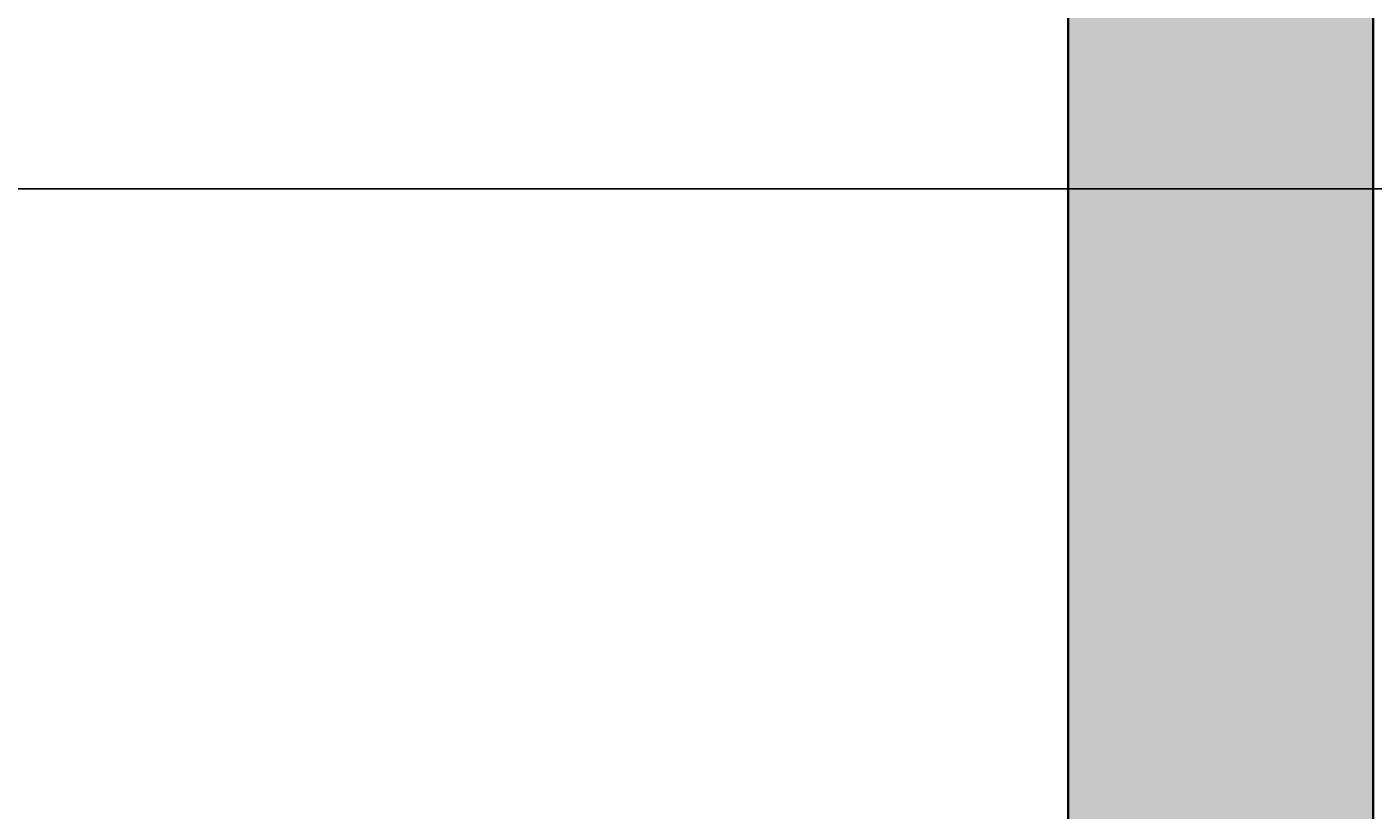
# Model space of a CAD drawing. Units: inches. Extents: x 1998 to 2588, y 1139 to 1977.
# Tile 13 of 134: x 2075 to 2115, y 1645 to 1668. Entities that reach past the tile are written whole.
import ezdxf

# ---------------------------------------------------------------- set-up
doc = ezdxf.new("R2010")
doc.units = ezdxf.units.IN
for name, color, linetype, lineweight in [('A-ANNO-DIMS', 2, 'Continuous', 18), ('A-WALL-PATT', 252, 'Continuous', 13), ('WALL', 200, 'Continuous', 35)]:
    doc.layers.add(name, color=color, linetype=linetype, lineweight=lineweight)
doc.styles.get("Standard").update_dxf_attribs({"font": 'arial.ttf'})
doc.dimstyles.get("Standard").update_dxf_attribs({"dimtxt": 0.18, "dimasz": 0.18, "dimexe": 0.18, "dimexo": 0.0625, "dimgap": 0.09, "dimtad": 0, "dimtih": 1, "dimtoh": 1, "dimdec": 4, "dimzin": 0, "dimdsep": 46, "dimtxsty": 'Standard', "dimcen": 0.09, "dimadec": 0, "dimazin": 0, "dimtfac": 1, "dimtdec": 4, "dimtofl": 0, "dimtmove": 0, "dimatfit": 3, "dimfxl": 1, "dimtolj": 1, "dimtzin": 0, "dimarcsym": 0})

# ---------------------------------------------------------------- blocks, each defined once
blk = doc.blocks.new('*D38')
at = {"layer": 'A-ANNO-DIMS', "color": 0, "lineweight": -2, "transparency": 16777216}
for p, q in [((2197.387, 1663.247), (1997.843, 1663.247)), ((1998.023, 1663.067), (1998.023, 1638.171)), ((1998.023, 1612.912), (1998.023, 1637.808)), ((2197.387, 1612.732), (1997.843, 1612.732))]:
    blk.add_line(p, q, dxfattribs=at)
at = {"layer": 'A-ANNO-DIMS', "color": 0, "transparency": 16777216}
for points in [[(1997.993, 1663.067), (1998.053, 1663.067), (1998.023, 1663.247)], [(1997.993, 1612.912), (1998.053, 1612.912), (1998.023, 1612.732)]]:
    blk.add_solid(points, dxfattribs=at)
at = {"layer": 'Defpoints', "color": 0, "transparency": 16777216}
for p in [(1998.023, 1663.247), (2197.45, 1663.247), (2197.45, 1612.732)]:
    blk.add_point(p, dxfattribs=at)
at = {"layer": 'A-ANNO-DIMS', "color": 0, "transparency": 16777216, "insert": (1998.023, 1637.99), "char_height": 0.18, "attachment_point": 5}
blk.add_mtext('\\A1;50.51', dxfattribs=at)
blk = doc.blocks.new('*D40')
at = {"layer": 'A-ANNO-DIMS', "color": 0, "lineweight": -2, "transparency": 16777216}
for p, q in [((2105.973, 1628.541), (2105.973, 1977.362)), ((2106.153, 1977.182), (2110.324, 1977.182)), ((2114.793, 1977.182), (2110.622, 1977.182)), ((2114.973, 1628.804), (2114.973, 1977.362))]:
    blk.add_line(p, q, dxfattribs=at)
at = {"layer": 'A-ANNO-DIMS', "color": 0, "transparency": 16777216}
for points in [[(2106.153, 1977.212), (2106.153, 1977.152), (2105.973, 1977.182)], [(2114.793, 1977.212), (2114.793, 1977.152), (2114.973, 1977.182)]]:
    blk.add_solid(points, dxfattribs=at)
at = {"layer": 'Defpoints', "color": 0, "transparency": 16777216}
for p in [(2114.973, 1977.182), (2114.973, 1628.742), (2105.973, 1628.478)]:
    blk.add_point(p, dxfattribs=at)
at = {"layer": 'A-ANNO-DIMS', "color": 0, "transparency": 16777216, "insert": (2110.473, 1977.182), "char_height": 0.18, "attachment_point": 5}
blk.add_mtext('\\A1;9', dxfattribs=at)

msp = doc.modelspace()

# ---------------------------------------------------------------- hatches: boundary and pattern name
at = {"layer": 'A-WALL-PATT'}
h = msp.add_hatch(color=256, dxfattribs=at)
h.dxf.hatch_style = 1
h.paths.add_polyline_path([(2527.4729, 1362.2324), (2510.9729, 1362.2324), (2510.9729, 1357.7324), (2518.4729, 1357.7324), (2518.4729, 1237.7324), (2503.1458, 1237.7324), (2503.1458, 1228.7324), (2527.4729, 1228.7324)])
h.paths.add_polyline_path([(2490.5682, 1362.2324), (2398.4729, 1362.2324), (2398.4729, 1357.7324), (2490.5682, 1357.7324)])
h.paths.add_polyline_path([(2224.9729, 1264.7324), (2222.9729, 1264.7324), (2222.9729, 1232.4125), (2341.4729, 1232.4125), (2341.4729, 1234.4125), (2224.9729, 1234.4125)])
h.paths.add_polyline_path([(2334.5332, 1273.7324), (2264.7638, 1273.7324), (2264.7638, 1269.5611, -0.043659), (2264.3413, 1264.7324), (2334.5332, 1264.7324)])
h.paths.add_polyline_path([(2236.9551, 1273.7324), (2234.4125, 1273.7324), (2234.4125, 1264.7324), (2236.9551, 1264.7324), (2236.9551, 1269.5611)])
h.paths.add_polyline_path([(2222.9729, 1293.2324), (2096.9729, 1293.2324), (2096.9729, 1345.0966), (2087.9729, 1345.0966), (2087.9729, 1284.2324), (2222.9729, 1284.2324), (2222.9729, 1285.137)])
h.paths.add_polyline_path([(2096.9729, 1458.7927), (2087.9729, 1458.7927), (2087.9729, 1417.7324), (2087.9729, 1413.2324), (2096.9729, 1413.2324), (2096.9729, 1417.7324)])
h.paths.add_polyline_path([(2096.9729, 1413.2324), (2087.9729, 1413.2324), (2087.9729, 1365.5012), (2096.9729, 1365.5012), (2096.9729, 1369.3358)])
h.paths.add_polyline_path([(2186.2943, 1417.7324), (2138.6074, 1417.7324), (2096.9729, 1417.7324), (2096.9729, 1413.2324), (2138.6074, 1413.2324), (2186.2943, 1413.2324)])
h.paths.add_polyline_path([(2181.4729, 1465.7324), (2176.9729, 1465.7324), (2176.9729, 1451.6434), (2181.4729, 1451.6434)])
h.paths.add_polyline_path([(2181.4729, 1422.1664), (2176.9729, 1422.1664), (2176.9729, 1417.7324), (2181.4729, 1417.7324)])
h.paths.add_polyline_path([(2063.9729, 1465.7324), (2087.9729, 1465.7324), (2087.9729, 1470.2324), (2059.4729, 1470.2324), (2059.4729, 1413.2324), (2087.9729, 1413.2324), (2087.9729, 1417.7324), (2063.9729, 1417.7324)])
h.paths.add_polyline_path([(2181.4729, 1755.2324), (2176.9729, 1755.2324), (2176.9729, 1748.6798), (2177.0513, 1748.6798), (2181.4729, 1748.6798)])
h.paths.add_polyline_path([(2227.4729, 1707.2324), (2220.4647, 1707.2324), (2220.4647, 1702.7324), (2222.9729, 1702.7324), (2222.9729, 1604.637), (2227.4729, 1604.637)])
h.paths.add_polyline_path([(2114.9729, 1702.7324), (2105.9729, 1702.7324), (2105.9729, 1628.4781, -0.0318759), (2110.1012, 1628.7416), (2114.9729, 1628.7416)])
h.paths.add_polyline_path([(2345.9729, 1739.3278), (2341.4729, 1739.3278), (2341.4729, 1647.5211), (2345.9729, 1647.5211)])
h.paths.add_polyline_path([(2350.6273, 1641.2324), (2345.9729, 1641.2324), (2345.9729, 1636.7324), (2350.6273, 1636.7324), (2350.6273, 1639.8729)])
h.paths.add_polyline_path([(2501.9729, 1641.2324), (2407.9729, 1641.2324), (2392.5005, 1641.2324), (2392.5005, 1639.8729), (2392.5005, 1636.7324), (2501.9729, 1636.7324)])
h.paths.add_polyline_path([(2510.9729, 1755.2324), (2501.9729, 1755.2324), (2501.9729, 1641.2324), (2510.9729, 1641.2324)])
h.paths.add_polyline_path([(2549.1786, 1641.2324), (2522.3775, 1641.2324), (2522.3775, 1636.7324), (2540.1786, 1636.7324), (2540.1786, 1480.7324), (2522.3775, 1480.7324), (2522.3775, 1476.2324), (2549.1786, 1476.2324)])
h.paths.add_polyline_path([(2498.1786, 1594.7324), (2407.9729, 1594.7324), (2407.9729, 1585.7324), (2416.9729, 1585.7324), (2489.1786, 1585.7324), (2489.1786, 1531.7324), (2416.9729, 1531.7324), (2407.9729, 1531.7324), (2407.9729, 1522.7324), (2498.1786, 1522.7324)])
h.paths.add_polyline_path([(2351.6437, 1480.7324), (2345.9729, 1480.7324), (2345.9729, 1476.2324), (2351.6437, 1476.2324), (2351.6437, 1477.5919)])
h.paths.add_polyline_path([(2501.9729, 1480.7324), (2498.1786, 1480.7324), (2407.9729, 1480.7324), (2393.5168, 1480.7324), (2393.5168, 1477.5919), (2393.5168, 1476.2324), (2501.9729, 1476.2324)])

# ---------------------------------------------------------------- linework, layer by layer
at = {"layer": 'WALL'}
for p, q in [((2105.9729, 1628.4781), (2105.9729, 1702.7324)), ((2114.9729, 1628.7416), (2114.9729, 1702.7324))]:
    msp.add_line(p, q, dxfattribs=at)

# ---------------------------------------------------------------- dimensions: what is measured, and where the dimension line sits
at = {"layer": 'A-ANNO-DIMS'}
dim = msp.add_linear_dim(base=(2114.9729, 1977.1824), p1=(2105.9729, 1628.4781), p2=(2114.9729, 1628.7416), dimstyle='Standard', override={"dimdec": 0, "dimlfac": 1, "dimrnd": 0, "dimzin": 0, "dimdsep": 46, "dimlunit": 2}, dxfattribs=at)
dim.commit()
dim.dimension.update_dxf_attribs({"geometry": '*D40', "text_midpoint": (2110.4729, 1977.1824)})
dim = msp.add_linear_dim(base=(1998.0229, 1663.2466), p1=(2197.4499, 1612.7324), p2=(2197.4499, 1663.2466), angle=90, dimstyle='Standard', override={"dimdec": 2, "dimlfac": 1, "dimrnd": 0, "dimzin": 0, "dimdsep": 46, "dimlunit": 2}, dxfattribs=at)
dim.commit()
dim.dimension.update_dxf_attribs({"geometry": '*D38', "text_midpoint": (1998.0229, 1637.9895)})

doc.saveas('drawing.dxf')
